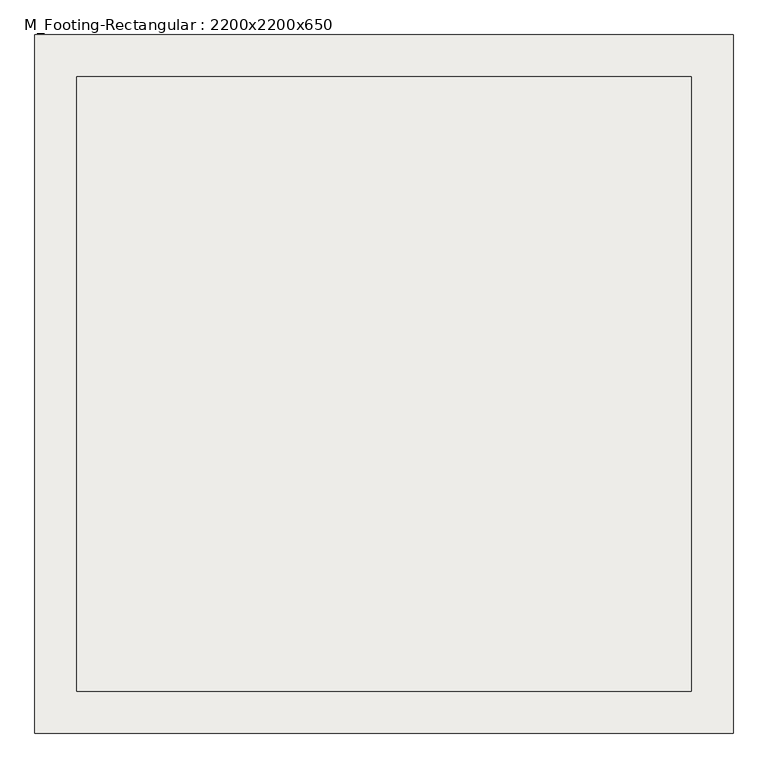
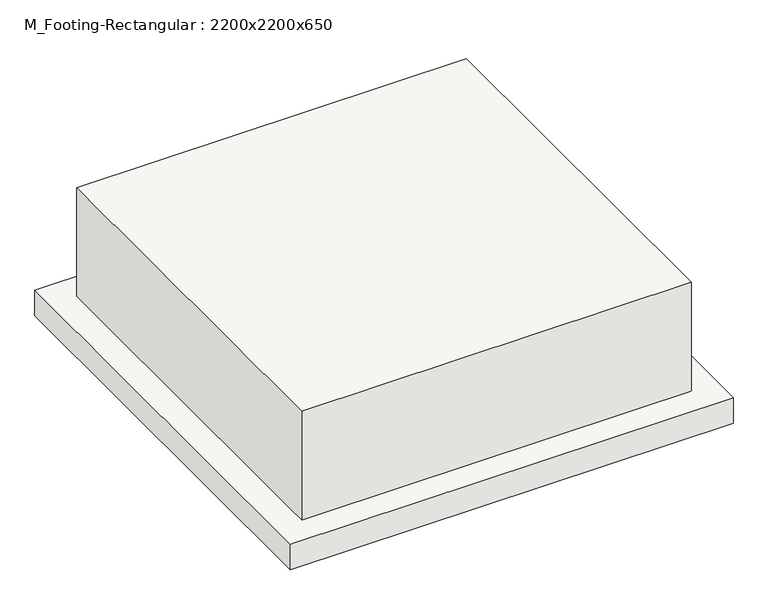
"""IFC4 building model written with IfcOpenShell, lengths in millimetres: slab geometry, M_Footing-Rectangular : 2200x2200x650."""

from ifc_helpers import new_model, si_unit, frame, origin, place, context, project, spatial, polyline, outline, extrude, source, transform, mapped, element, save


def m_footing_rectangular_2200x2200x650_5a9dd948(model_context):
    return source(origin(), model_context, "Body", "SweptSolid", [
        extrude(outline(polyline([(1250.0, 1250.0), (1250.0, -1250.0), (-1250.0, -1250.0), (-1250.0, 1250.0), (1250.0, 1250.0)])), frame((0.0, 0.0, -802.4), z_axis=(0.0, 0.0, 1.0), x_axis=(1.0, 0.0, 0.0)), (0.0, 0.0, 1.0), 152.4),
        extrude(outline(polyline([(1100.0, 1100.0), (1100.0, -1100.0), (-1100.0, -1100.0), (-1100.0, 1100.0), (1100.0, 1100.0)])), frame((0.0, 0.0, -650.0), z_axis=(0.0, 0.0, 1.0), x_axis=(1.0, 0.0, 0.0)), (0.0, 0.0, 1.0), 650.0),
    ])


if __name__ == "__main__":
    model = new_model("IFC4")
    model_context = context("Model", 3, world=origin())
    ifc_project = project(units=[si_unit("LENGTHUNIT", "METRE", prefix="MILLI")], contexts=[model_context])
    site = spatial("IfcSite", under=ifc_project)
    building = spatial("IfcBuilding", under=site)
    placement = place(None, origin())
    m_footing_rectangular_2200x2200x650_shape = m_footing_rectangular_2200x2200x650_5a9dd948(model_context)
    element("IfcSlab", 1, ObjectType="M_Footing-Rectangular : 2200x2200x650", at=placement, inside=building, context=model_context, shape_type="MappedRepresentation", body=[
        mapped(m_footing_rectangular_2200x2200x650_shape, transform((0.0, 0.0, 0.0), x_axis=(1.0, 0.0, 0.0), y_axis=(0.0, 1.0, 0.0), z_axis=(0.0, 0.0, 1.0))),
    ])
    save(model, "model.ifc")

# Revit data of these elements
# Type "M_Footing-Rectangular : 2200x2200x650"
#   Width = 2200 mm
#   Length = 2200 mm
#   Foundation Thickness = 650 mm
#   Structural Material [instance default] = Concrete, Cast-in-Place gray
#   Assembly Code = ""
# Element 1 (IfcSlab, "M_Footing-Rectangular : 2200x2200x650")
#   Materials on its faces: "Concrete, Cast-in-Place gray"
# Materials
#   "Concrete, Cast-in-Place gray": class "Concrete", colour RGB 192 192 192, transparency 0, Description = "Cast-in-place concrete", Cost = 0
